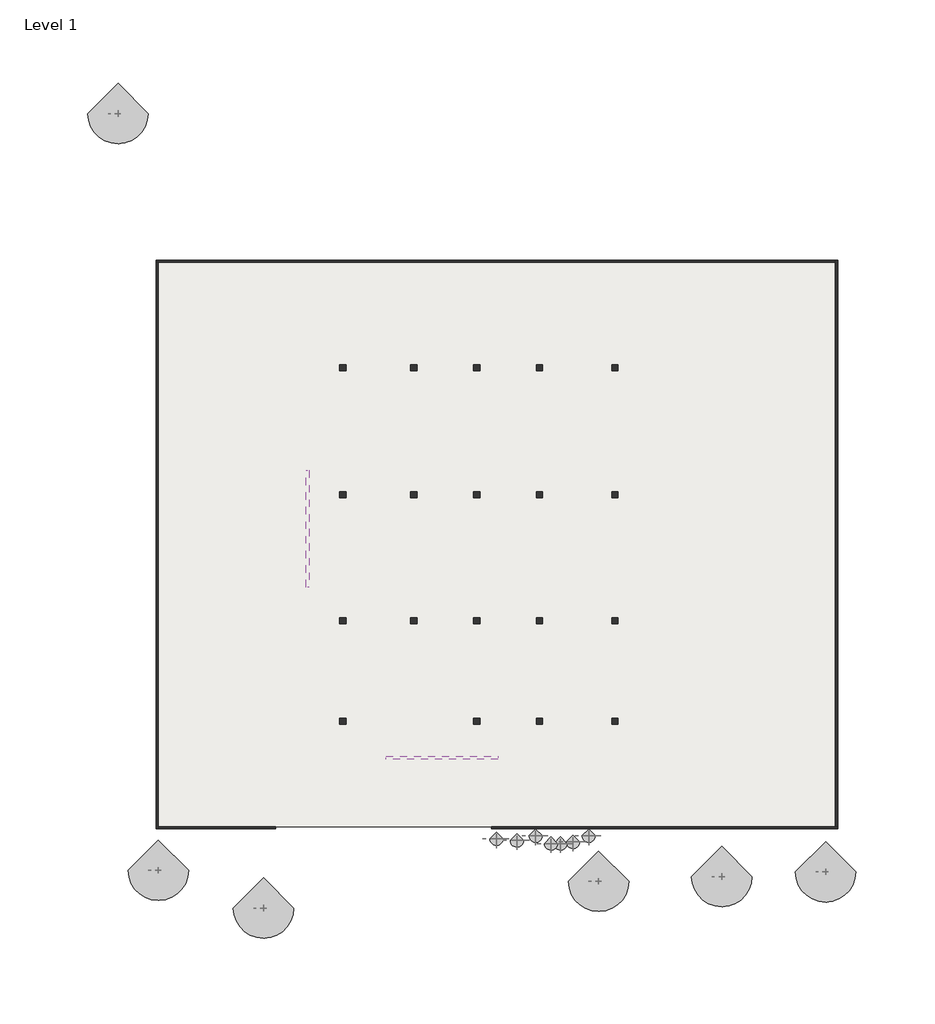
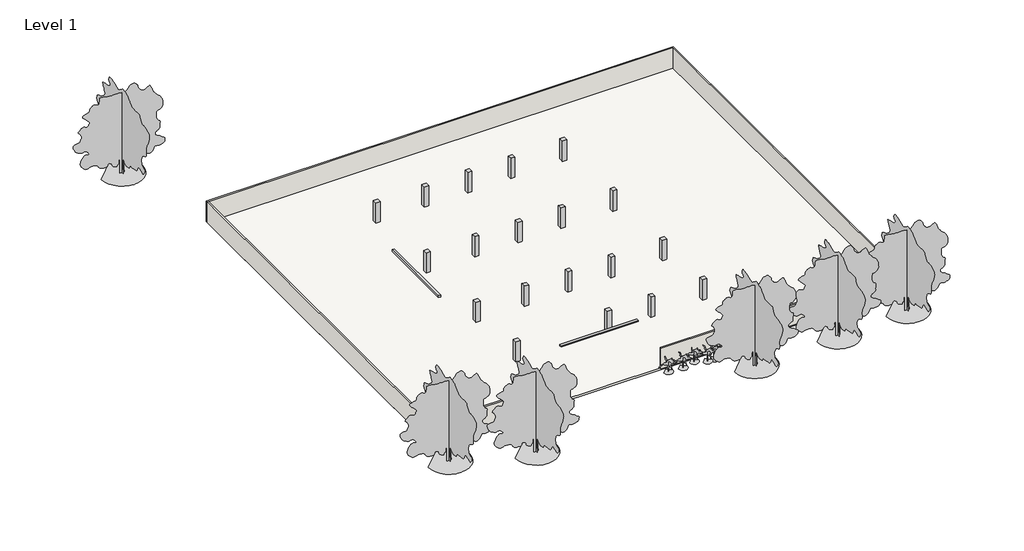
# One storey: 19 columns, 13 geographic elements, 4 walls, 2 proxies, 1 slab.
"""IFC4 building model written with IfcOpenShell, lengths in millimetres."""

from ifc_helpers import new_model, si_unit, frame, origin, place, context, project, spatial, polyline, outline, extrude, faceted_brep, transform, mapped, element, save
from components import generic_models_12_generic_models_12_c9051349, generic_models_23_generic_models_23_92ef9671, column_c091e905, rpc_tree_deciduous_scarlet_oak_42_9b182cbb, rpc_tree_tropical_australian_tree_furn_6_77f1a640

model = new_model("IFC4")

# Units and contexts
model_context = context("Model", 3, world=origin())
ifc_project = project(units=[si_unit("LENGTHUNIT", "METRE", prefix="MILLI")], contexts=[model_context])

# Site, building, storey
site = spatial("IfcSite", under=ifc_project)
building = spatial("IfcBuilding", under=site)
storey = spatial("IfcBuildingStorey", under=building, Name="Level 1", Elevation=0.0)

# Proxies
placement = place(None, origin())
generic_models_12_generic_models_12_shape = generic_models_12_generic_models_12_c9051349(model_context)
element("IfcBuildingElementProxy", 1, Name="Generic Models 12 : Generic Models 12", ObjectType="Generic Models 12 : Generic Models 12", at=placement, inside=storey, context=model_context, shape_type="MappedRepresentation", body=[
    mapped(generic_models_12_generic_models_12_shape, transform((0.0, 0.0, 0.0), x_axis=(1.0, 0.0, 0.0), y_axis=(0.0, 1.0, 0.0), z_axis=(0.0, 0.0, 1.0))),
])
generic_models_23_generic_models_23_shape = generic_models_23_generic_models_23_92ef9671(model_context)
element("IfcBuildingElementProxy", 2, Name="Generic Models 23 : Generic Models 23", ObjectType="Generic Models 23 : Generic Models 23", at=placement, inside=storey, context=model_context, shape_type="MappedRepresentation", body=[
    mapped(generic_models_23_generic_models_23_shape, transform((0.0, 0.0, 0.0), x_axis=(1.0, 0.0, 0.0), y_axis=(0.0, 1.0, 0.0), z_axis=(0.0, 0.0, 1.0))),
])

# Columns
column_shape = column_c091e905(model_context)
element("IfcColumn", 3, ObjectType="Rectangular Column : 24\" x 24\"", at=placement, inside=storey, context=model_context, shape_type="MappedRepresentation", body=[
    mapped(column_shape, transform((-11814.7904228, 16893.6152028, 0.0), x_axis=(1.0, 0.0, 0.0), y_axis=(0.0, 1.0, 0.0), z_axis=(0.0, 0.0, 1.0))),
])
element("IfcColumn", 4, ObjectType="Rectangular Column : 24\" x 24\"", at=placement, inside=storey, context=model_context, shape_type="MappedRepresentation", body=[
    mapped(column_shape, transform((-4956.7904228, 16893.6152028, 0.0), x_axis=(1.0, 0.0, 0.0), y_axis=(0.0, 1.0, 0.0), z_axis=(0.0, 0.0, 1.0))),
])
element("IfcColumn", 5, ObjectType="Rectangular Column : 24\" x 24\"", at=placement, inside=storey, context=model_context, shape_type="MappedRepresentation", body=[
    mapped(column_shape, transform((1139.2095772, 16893.6152028, 0.0), x_axis=(1.0, 0.0, 0.0), y_axis=(0.0, 1.0, 0.0), z_axis=(0.0, 0.0, 1.0))),
])
element("IfcColumn", 6, ObjectType="Rectangular Column : 24\" x 24\"", at=placement, inside=storey, context=model_context, shape_type="MappedRepresentation", body=[
    mapped(column_shape, transform((7235.2095772, 16893.6152028, 0.0), x_axis=(1.0, 0.0, 0.0), y_axis=(0.0, 1.0, 0.0), z_axis=(0.0, 0.0, 1.0))),
])
element("IfcColumn", 7, ObjectType="Rectangular Column : 24\" x 24\"", at=placement, inside=storey, context=model_context, shape_type="MappedRepresentation", body=[
    mapped(column_shape, transform((14550.4095772, 16893.6152028, 0.0), x_axis=(1.0, 0.0, 0.0), y_axis=(0.0, 1.0, 0.0), z_axis=(0.0, 0.0, 1.0))),
])
element("IfcColumn", 8, ObjectType="Rectangular Column : 24\" x 24\"", at=placement, inside=storey, context=model_context, shape_type="MappedRepresentation", body=[
    mapped(column_shape, transform((14550.4095772, 4586.3482288, 0.0), x_axis=(1.0, 0.0, 0.0), y_axis=(0.0, 1.0, 0.0), z_axis=(0.0, 0.0, 1.0))),
])
element("IfcColumn", 9, ObjectType="Rectangular Column : 24\" x 24\"", at=placement, inside=storey, context=model_context, shape_type="MappedRepresentation", body=[
    mapped(column_shape, transform((7235.2095772, 4586.3482288, 0.0), x_axis=(1.0, 0.0, 0.0), y_axis=(0.0, 1.0, 0.0), z_axis=(0.0, 0.0, 1.0))),
])
element("IfcColumn", 10, ObjectType="Rectangular Column : 24\" x 24\"", at=placement, inside=storey, context=model_context, shape_type="MappedRepresentation", body=[
    mapped(column_shape, transform((1139.2095772, 4586.3482288, 0.0), x_axis=(1.0, 0.0, 0.0), y_axis=(0.0, 1.0, 0.0), z_axis=(0.0, 0.0, 1.0))),
])
element("IfcColumn", 11, ObjectType="Rectangular Column : 24\" x 24\"", at=placement, inside=storey, context=model_context, shape_type="MappedRepresentation", body=[
    mapped(column_shape, transform((-4956.7904228, 4586.3482288, 0.0), x_axis=(1.0, 0.0, 0.0), y_axis=(0.0, 1.0, 0.0), z_axis=(0.0, 0.0, 1.0))),
])
element("IfcColumn", 12, ObjectType="Rectangular Column : 24\" x 24\"", at=placement, inside=storey, context=model_context, shape_type="MappedRepresentation", body=[
    mapped(column_shape, transform((-11814.7904228, 4586.3482288, 0.0), x_axis=(1.0, 0.0, 0.0), y_axis=(0.0, 1.0, 0.0), z_axis=(0.0, 0.0, 1.0))),
])
element("IfcColumn", 13, ObjectType="Rectangular Column : 24\" x 24\"", at=placement, inside=storey, context=model_context, shape_type="MappedRepresentation", body=[
    mapped(column_shape, transform((-11814.7904228, -7605.6517712, 0.0), x_axis=(1.0, 0.0, 0.0), y_axis=(0.0, 1.0, 0.0), z_axis=(0.0, 0.0, 1.0))),
])
element("IfcColumn", 14, ObjectType="Rectangular Column : 24\" x 24\"", at=placement, inside=storey, context=model_context, shape_type="MappedRepresentation", body=[
    mapped(column_shape, transform((-4956.7904228, -7605.6517712, 0.0), x_axis=(1.0, 0.0, 0.0), y_axis=(0.0, 1.0, 0.0), z_axis=(0.0, 0.0, 1.0))),
])
element("IfcColumn", 15, ObjectType="Rectangular Column : 24\" x 24\"", at=placement, inside=storey, context=model_context, shape_type="MappedRepresentation", body=[
    mapped(column_shape, transform((1139.2095772, -7605.6517712, 0.0), x_axis=(1.0, 0.0, 0.0), y_axis=(0.0, 1.0, 0.0), z_axis=(0.0, 0.0, 1.0))),
])
element("IfcColumn", 16, ObjectType="Rectangular Column : 24\" x 24\"", at=placement, inside=storey, context=model_context, shape_type="MappedRepresentation", body=[
    mapped(column_shape, transform((7235.2095772, -7605.6517712, 0.0), x_axis=(1.0, 0.0, 0.0), y_axis=(0.0, 1.0, 0.0), z_axis=(0.0, 0.0, 1.0))),
])
element("IfcColumn", 17, ObjectType="Rectangular Column : 24\" x 24\"", at=placement, inside=storey, context=model_context, shape_type="MappedRepresentation", body=[
    mapped(column_shape, transform((14550.4095772, -7605.6517712, 0.0), x_axis=(1.0, 0.0, 0.0), y_axis=(0.0, 1.0, 0.0), z_axis=(0.0, 0.0, 1.0))),
])
element("IfcColumn", 18, ObjectType="Rectangular Column : 24\" x 24\"", at=placement, inside=storey, context=model_context, shape_type="MappedRepresentation", body=[
    mapped(column_shape, transform((14550.4095772, -17359.2517712, 0.0), x_axis=(1.0, 0.0, 0.0), y_axis=(0.0, 1.0, 0.0), z_axis=(0.0, 0.0, 1.0))),
])
element("IfcColumn", 19, ObjectType="Rectangular Column : 24\" x 24\"", at=placement, inside=storey, context=model_context, shape_type="MappedRepresentation", body=[
    mapped(column_shape, transform((7235.2095772, -17359.2517712, 0.0), x_axis=(1.0, 0.0, 0.0), y_axis=(0.0, 1.0, 0.0), z_axis=(0.0, 0.0, 1.0))),
])
element("IfcColumn", 20, ObjectType="Rectangular Column : 24\" x 24\"", at=placement, inside=storey, context=model_context, shape_type="MappedRepresentation", body=[
    mapped(column_shape, transform((1139.2095772, -17359.2517712, 0.0), x_axis=(1.0, 0.0, 0.0), y_axis=(0.0, 1.0, 0.0), z_axis=(0.0, 0.0, 1.0))),
])
element("IfcColumn", 21, ObjectType="Rectangular Column : 24\" x 24\"", at=placement, inside=storey, context=model_context, shape_type="MappedRepresentation", body=[
    mapped(column_shape, transform((-11814.7904228, -17359.2517712, 0.0), x_axis=(1.0, 0.0, 0.0), y_axis=(0.0, 1.0, 0.0), z_axis=(0.0, 0.0, 1.0))),
])

# Geographic elements
rpc_tree_deciduous_scarlet_oak_42_shape = rpc_tree_deciduous_scarlet_oak_42_9b182cbb(model_context)
element("IfcGeographicElement", 22, ObjectType="RPC Tree - Deciduous : Scarlet Oak - 42'", at=placement, inside=storey, context=model_context, shape_type="MappedRepresentation", body=[
    mapped(rpc_tree_deciduous_scarlet_oak_42_shape, transform((34959.3592352, -31938.09573, 0.0), x_axis=(1.0, 0.0, 0.0), y_axis=(0.0, 1.0, 0.0), z_axis=(0.0, 0.0, 1.0))),
])
element("IfcGeographicElement", 23, ObjectType="RPC Tree - Deciduous : Scarlet Oak - 42'", at=placement, inside=storey, context=model_context, shape_type="MappedRepresentation", body=[
    mapped(rpc_tree_deciduous_scarlet_oak_42_shape, transform((24900.9592352, -32395.29573, 0.0), x_axis=(1.0, 0.0, 0.0), y_axis=(0.0, 1.0, 0.0), z_axis=(0.0, 0.0, 1.0))),
])
element("IfcGeographicElement", 24, ObjectType="RPC Tree - Deciduous : Scarlet Oak - 42'", at=placement, inside=storey, context=model_context, shape_type="MappedRepresentation", body=[
    mapped(rpc_tree_deciduous_scarlet_oak_42_shape, transform((12968.161926, -32852.49573, 0.0), x_axis=(1.0, 0.0, 0.0), y_axis=(0.0, 1.0, 0.0), z_axis=(0.0, 0.0, 1.0))),
])
element("IfcGeographicElement", 25, ObjectType="RPC Tree - Deciduous : Scarlet Oak - 42'", at=placement, inside=storey, context=model_context, shape_type="MappedRepresentation", body=[
    mapped(rpc_tree_deciduous_scarlet_oak_42_shape, transform((-19512.4693425, -35443.29573, 0.0), x_axis=(1.0, 0.0, 0.0), y_axis=(0.0, 1.0, 0.0), z_axis=(0.0, 0.0, 1.0))),
])
element("IfcGeographicElement", 26, ObjectType="RPC Tree - Deciduous : Scarlet Oak - 42'", at=placement, inside=storey, context=model_context, shape_type="MappedRepresentation", body=[
    mapped(rpc_tree_deciduous_scarlet_oak_42_shape, transform((-29709.0407648, -31785.69573, 0.0), x_axis=(1.0, 0.0, 0.0), y_axis=(0.0, 1.0, 0.0), z_axis=(0.0, 0.0, 1.0))),
])
element("IfcGeographicElement", 27, ObjectType="RPC Tree - Deciduous : Scarlet Oak - 42'", at=placement, inside=storey, context=model_context, shape_type="MappedRepresentation", body=[
    mapped(rpc_tree_deciduous_scarlet_oak_42_shape, transform((-33620.6407648, 41518.70427, 0.0), x_axis=(1.0, 0.0, 0.0), y_axis=(0.0, 1.0, 0.0), z_axis=(0.0, 0.0, 1.0))),
])
rpc_tree_tropical_australian_tree_furn_6_shape = rpc_tree_tropical_australian_tree_furn_6_77f1a640(model_context)
element("IfcGeographicElement", 28, ObjectType="RPC Tree - Tropical : Australian Tree Furn - 6'", at=placement, inside=storey, context=model_context, shape_type="MappedRepresentation", body=[
    mapped(rpc_tree_tropical_australian_tree_furn_6_shape, transform((3056.9592352, -28737.69573, 0.0), x_axis=(1.0, 0.0, 0.0), y_axis=(0.0, 1.0, 0.0), z_axis=(0.0, 0.0, 1.0))),
])
element("IfcGeographicElement", 29, ObjectType="RPC Tree - Tropical : Australian Tree Furn - 6'", at=placement, inside=storey, context=model_context, shape_type="MappedRepresentation", body=[
    mapped(rpc_tree_tropical_australian_tree_furn_6_shape, transform((5038.1592352, -28890.09573, 0.0), x_axis=(1.0, 0.0, 0.0), y_axis=(0.0, 1.0, 0.0), z_axis=(0.0, 0.0, 1.0))),
])
element("IfcGeographicElement", 30, ObjectType="RPC Tree - Tropical : Australian Tree Furn - 6'", at=placement, inside=storey, context=model_context, shape_type="MappedRepresentation", body=[
    mapped(rpc_tree_tropical_australian_tree_furn_6_shape, transform((6866.9592352, -28432.89573, 0.0), x_axis=(1.0, 0.0, 0.0), y_axis=(0.0, 1.0, 0.0), z_axis=(0.0, 0.0, 1.0))),
])
element("IfcGeographicElement", 31, ObjectType="RPC Tree - Tropical : Australian Tree Furn - 6'", at=placement, inside=storey, context=model_context, shape_type="MappedRepresentation", body=[
    mapped(rpc_tree_tropical_australian_tree_furn_6_shape, transform((9259.761926, -29194.89573, 0.0), x_axis=(1.0, 0.0, 0.0), y_axis=(0.0, 1.0, 0.0), z_axis=(0.0, 0.0, 1.0))),
])
element("IfcGeographicElement", 32, ObjectType="RPC Tree - Tropical : Australian Tree Furn - 6'", at=placement, inside=storey, context=model_context, shape_type="MappedRepresentation", body=[
    mapped(rpc_tree_tropical_australian_tree_furn_6_shape, transform((8345.361926, -29194.89573, 0.0), x_axis=(1.0, 0.0, 0.0), y_axis=(0.0, 1.0, 0.0), z_axis=(0.0, 0.0, 1.0))),
])
element("IfcGeographicElement", 33, ObjectType="RPC Tree - Tropical : Australian Tree Furn - 6'", at=placement, inside=storey, context=model_context, shape_type="MappedRepresentation", body=[
    mapped(rpc_tree_tropical_australian_tree_furn_6_shape, transform((10478.961926, -29042.49573, 0.0), x_axis=(1.0, 0.0, 0.0), y_axis=(0.0, 1.0, 0.0), z_axis=(0.0, 0.0, 1.0))),
])
element("IfcGeographicElement", 34, ObjectType="RPC Tree - Tropical : Australian Tree Furn - 6'", at=placement, inside=storey, context=model_context, shape_type="MappedRepresentation", body=[
    mapped(rpc_tree_tropical_australian_tree_furn_6_shape, transform((12002.961926, -28432.89573, 0.0), x_axis=(1.0, 0.0, 0.0), y_axis=(0.0, 1.0, 0.0), z_axis=(0.0, 0.0, 1.0))),
])

# Slab
element("IfcSlab", 35, ObjectType="Generic - 12\"", at=placement, inside=storey, context=model_context, shape_type="SweptSolid", body=[
    extrude(outline(polyline([(35924.5592352, 27091.50427), (35924.5592352, -27569.29573), (-29709.0407648, -27569.29573), (-29709.0407648, 27091.50427), (35924.5592352, 27091.50427)])), frame((0.0, 0.0, -304.8), z_axis=(0.0, 0.0, 1.0), x_axis=(1.0, 0.0, 0.0)), (0.0, 0.0, 1.0), 304.8),
])

# Walls
element("IfcWall", 36, ObjectType="Generic - 8\"", at=placement, inside=storey, context=model_context, shape_type="Brep", body=[
    faceted_brep([(-29912.2407648, 27091.50427, 0.0), (-29709.0407648, 27091.50427, 0.0), (35924.5592352, 27091.50427, 0.0), (35924.5592352, 27091.50427, 3048.0), (-29709.0407648, 27091.50427, 3048.0), (-29912.2407648, 27091.50427, 3048.0), (-29912.2407648, 27294.70427, 0.0), (-29912.2407648, 27294.70427, 3048.0), (35924.5592352, 27294.70427, 3048.0), (35924.5592352, 27294.70427, 0.0)], [[[0, 1, 2, 3, 4, 5]], [[6, 7, 8, 9]], [[2, 1, 0, 6, 9]], [[5, 4, 3, 8, 7]], [[0, 5, 7, 6]], [[3, 2, 9, 8]]]),
])
element("IfcWall", 37, ObjectType="Generic - 8\"", at=placement, inside=storey, context=model_context, shape_type="Brep", body=[
    faceted_brep([(-29709.0407648, -27772.49573, 0.0), (-29709.0407648, -27569.29573, 0.0), (-29709.0407648, 27091.50427, 0.0), (-29709.0407648, 27091.50427, 3048.0), (-29709.0407648, -27569.29573, 3048.0), (-29709.0407648, -27772.49573, 3048.0), (-29912.2407648, -27772.49573, 0.0), (-29912.2407648, -27772.49573, 3048.0), (-29912.2407648, 27091.50427, 3048.0), (-29912.2407648, 27091.50427, 0.0)], [[[0, 1, 2, 3, 4, 5]], [[6, 7, 8, 9]], [[2, 1, 0, 6, 9]], [[5, 4, 3, 8, 7]], [[0, 5, 7, 6]], [[3, 2, 9, 8]]]),
])
element("IfcWall", 38, ObjectType="Generic - 8\"", at=placement, inside=storey, context=model_context, shape_type="Brep", body=[
    faceted_brep([(-29709.0407648, -27569.29573, 0.0), (-29709.0407648, -27569.29573, 3048.0), (-18326.913548, -27569.29573, 3048.0), (-18326.913548, -27569.29573, 0.0), (-29709.0407648, -27772.49573, 3048.0), (-29709.0407648, -27772.49573, 0.0), (-18326.913548, -27772.49573, 0.0), (-18326.913548, -27772.49573, 3048.0)], [[[0, 1, 2, 3]], [[4, 5, 6, 7]], [[5, 0, 3, 6]], [[1, 4, 7, 2]], [[1, 0, 5, 4]], [[3, 2, 7, 6]]]),
    faceted_brep([(36127.7592352, -27569.29573, 3048.0), (36127.7592352, -27569.29573, 0.0), (35924.5592352, -27569.29573, 0.0), (2560.7052415, -27569.29573, 0.0), (2560.7052415, -27569.29573, 3048.0), (35924.5592352, -27569.29573, 3048.0), (36127.7592352, -27772.49573, 0.0), (36127.7592352, -27772.49573, 3048.0), (2560.7052415, -27772.49573, 3048.0), (2560.7052415, -27772.49573, 0.0)], [[[0, 1, 2, 3, 4, 5]], [[6, 7, 8, 9]], [[1, 6, 9, 3, 2]], [[7, 0, 5, 4, 8]], [[1, 0, 7, 6]], [[4, 3, 9, 8]]]),
])
element("IfcWall", 39, ObjectType="Generic - 8\"", at=placement, inside=storey, context=model_context, shape_type="Brep", body=[
    faceted_brep([(35924.5592352, 27294.70427, 0.0), (35924.5592352, 27091.50427, 0.0), (35924.5592352, -27569.29573, 0.0), (35924.5592352, -27569.29573, 3048.0), (35924.5592352, 27091.50427, 3048.0), (35924.5592352, 27294.70427, 3048.0), (36127.7592352, 27294.70427, 0.0), (36127.7592352, 27294.70427, 3048.0), (36127.7592352, -27569.29573, 3048.0), (36127.7592352, -27569.29573, 0.0)], [[[0, 1, 2, 3, 4, 5]], [[6, 7, 8, 9]], [[2, 1, 0, 6, 9]], [[5, 4, 3, 8, 7]], [[0, 5, 7, 6]], [[3, 2, 9, 8]]]),
])

save(model, "model.ifc")

# Revit data of these elements
# Grids (mm)
#   "1": line (-11814.79, -17359.252) -> (-11814.79, 16893.615)
#   "2": line (-11814.79, -17359.252) -> (18665.21, -17359.252)
#   "3": line (18665.21, -7605.652) -> (-11814.79, -7605.652)
#   "4": line (18665.21, 4586.348) -> (-11814.79, 4586.348)
#   "5": line (17996.623, 16893.615) -> (-11814.79, 16893.615)
#   "6": line (-4956.79, 16893.615) -> (-4956.79, -17359.252)
#   "7": line (1139.21, -17359.252) -> (1139.21, 16893.615)
#   "8": line (7235.21, -17359.252) -> (7235.21, 16893.615)
#   "9": line (14550.41, -17359.252) -> (14550.41, 16893.615)
# Type "Rectangular Column : 24\" x 24\""
#   Assembly Code = "B1010200"
#   Depth = 2' - 0"
#   Offset Base = 0' - 0"
#   Offset Top = 0' - 0"
#   Width = 2' - 0"
#   Material = none
# Type "RPC Tree - Deciduous : Scarlet Oak - 42'"
#   built-in parameter 1005198 = "{2, 15},{39, RPC-16-G0FB-J5PX-0LX6-U000-ST1L-LVER-AU},{1, 0},{1, 0},{2, 13},{1, 8},{5, Color},{1, 0},{1, 0},{3, 0.8},{3, 0.8},{3, 0.8},{1, 8},{7, BBoxMin},{1, 0},{1, 0},{1, 0},{1, 0},{1, 0},{1, 8},{7, BBoxMax},{1, 0},{1, 0},{1, 0},{1, 0},{1, 0},{2, 11},{9, RPCTypeId},{1, 0},{1, 0},{39, RPC-16-G0FB-J5PX-0LX6-U000-ST1L-LVER-AU},{1, 6},{14, RPCPlantHeight},{1, 0},{1, 0},{2, 42},{2, 11},{7, keyword},{1, 0},{1, 0},{34, :RPCs:Trees [General]:Geometry:RPC},{2, 11},{8, category},{1, 0},{1, 0},{15, Trees [General]},{2, 11},{12, LocalizedUID},{1, 0},{1, 0},{11, Scarlet_Oak},{2, 14},{6, Height},{1, 0},{1, 0},{2, 42},{1, 2},{16, Cast Reflections},{1, 0},{1, 0},{1, 0},{1, 2},{12, Cast Shadows},{1, 0},{1, 0},{1, 1},{1, 2},{9, Lock View},{1, 0},{1, 0},{1, 0},{1, 4},{5, ViewC},{1, 0},{1, 0},{1, 0},{21, assetlibrary_base.fbx},{1, 5},"
#   built-in parameter 1005195 = "RPC-16-G0FB-J5PX-0LX6-U000-ST1L-LVER-AU"
#   Type Comments = "Scarlet Oak"
#   Assembly Code = "G2050500"
#   Height = 42' - 0"
#   Default Elevation = 0
# Type "RPC Tree - Tropical : Australian Tree Furn - 6'"
#   built-in parameter 1005198 = "{2, 15},{39, RPC-16-FVCN-UWG0-AP53-A000-ST1L-LVER-AU},{1, 0},{1, 0},{2, 13},{1, 8},{5, Color},{1, 0},{1, 0},{3, 0.8},{3, 0.8},{3, 0.8},{1, 8},{7, BBoxMin},{1, 0},{1, 0},{1, 0},{1, 0},{1, 0},{1, 8},{7, BBoxMax},{1, 0},{1, 0},{1, 0},{1, 0},{1, 0},{2, 11},{9, RPCTypeId},{1, 0},{1, 0},{39, RPC-16-FVCN-UWG0-AP53-A000-ST1L-LVER-AU},{1, 6},{14, RPCPlantHeight},{1, 0},{1, 0},{1, 6},{2, 11},{7, keyword},{1, 0},{1, 0},{35, :RPCs:Trees [Tropical]:Geometry:RPC},{2, 11},{8, category},{1, 0},{1, 0},{16, Trees [Tropical]},{2, 11},{12, LocalizedUID},{1, 0},{1, 0},{20, Australian Tree Fern},{2, 14},{6, Height},{1, 0},{1, 0},{1, 6},{1, 2},{16, Cast Reflections},{1, 0},{1, 0},{1, 0},{1, 2},{12, Cast Shadows},{1, 0},{1, 0},{1, 1},{1, 2},{9, Lock View},{1, 0},{1, 0},{1, 0},{1, 4},{5, ViewC},{1, 0},{1, 0},{1, 0},{21, assetlibrary_base.fbx},{1, 5},"
#   built-in parameter 1005195 = "RPC-16-FVCN-UWG0-AP53-A000-ST1L-LVER-AU"
#   Type Comments = "Australian Tree Furn"
#   Assembly Code = "G2050500"
#   Height = 6' - 0"
#   Plan Symbol = element 363555
#   Default Elevation = 0
# Type "Generic - 12\""
#   Assembly Code = "B1010"
#   Function = 0
#   Layers, outside or top first: 1' - 0" no material (function 1)
# Type "Generic - 8\""
#   Assembly Code = "B2010"
#   Layers, outside or top first: 0' - 8" no material (function 1)
# Element 1 (IfcBuildingElementProxy, "Generic Models 12 : Generic Models 12")
#   Phase Created = New Construction
# Element 2 (IfcBuildingElementProxy, "Generic Models 23 : Generic Models 23")
#   Phase Created = New Construction
# Elements 3, 4, 5, 6, 7, 8, 9, 10, 11, 12, 13, 14, 15, 16, 17, 18, 19, 20, 21 (IfcColumn, "Rectangular Column : 24\" x 24\"")
#   Phase Created = New Construction
# Elements 22, 23, 24, 25, 26, 27 (IfcGeographicElement, "RPC Tree - Deciduous : Scarlet Oak - 42'")
#   Phase Created = New Construction
# Elements 28, 29, 30, 31, 32, 33, 34 (IfcGeographicElement, "RPC Tree - Tropical : Australian Tree Furn - 6'")
#   Phase Created = New Construction
# Element 35 (IfcSlab, "Generic - 12\"")
#   Height Offset From Level = 0' - 0"
#   Phase Created = New Construction
#   Materials on its faces: "Default Floor"
# Elements 36, 37, 38, 39 (IfcWall, "Generic - 8\"")
#   Top Offset = 0' - 0"
#   Base Offset = 0' - 0"
#   Unconnected Height = 10' - 0"
#   wall height = 10' - 0"
#   Phase Created = New Construction
#   Base Constraint = Level 1
#   Materials on its faces: "Default Wall"
# Materials
#   "Default Floor": colour RGB 128 128 128, transparency 0
#   "Default Wall": colour RGB 128 128 128, transparency 0
